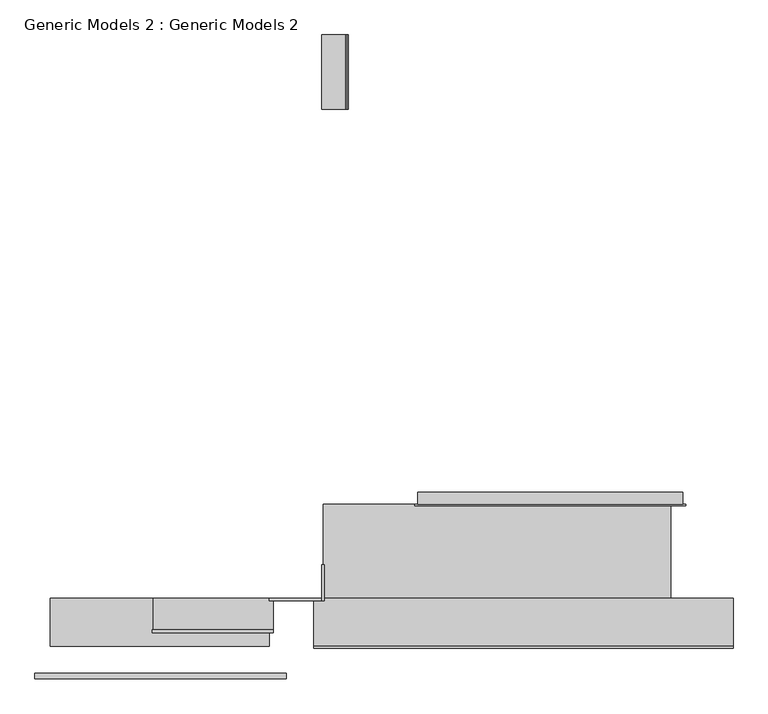
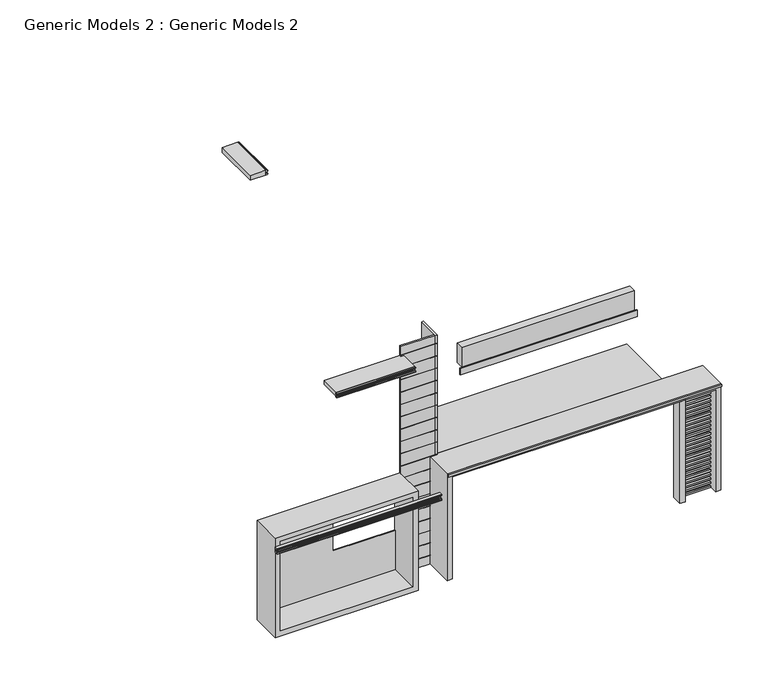
"""IFC4 building model written with IfcOpenShell, lengths in millimetres: proxy geometry, Generic Models 2 : Generic Models 2."""

from ifc_helpers import new_model, si_unit, point, frame, frame_2d, origin, place, context, project, spatial, polyline, circle_curve, trimmed, segment, composite_curve, outline, extrude, faceted_brep, source, transform, mapped, element, save


def generic_models_2_generic_models_2_638b9eba(model_context):
    return source(origin(), model_context, "Body", "SolidModel", [
        extrude(outline(polyline([(-7758.4277226, -3207.8444793), (-7758.4277226, -4630.2444793), (-7759.7175664, -4630.2444793), (-7759.7175664, -3207.8444793), (-7758.4277226, -3207.8444793)])), frame((0.0, 0.0, 6031.309375), z_axis=(0.0, 0.0, 1.0), x_axis=(1.0, 0.0, 0.0)), (0.0, 0.0, 1.0), 28.178125),
        extrude(outline(composite_curve([segment(polyline([(6121.4, -7759.7175664), (6059.4875, -7759.7175664), (6059.4875, -7747.0175664)]), True, "CONTINUOUS"), segment(trimmed(circle_curve(frame_2d((6072.1875, -7747.0175664)), 12.7), [point((6059.4875, -7747.0175664))], [point((6072.1875, -7734.3175664))], False, "CARTESIAN"), True, "CONTINUOUS"), segment(polyline([(6072.1875, -7734.3175664), (6083.3, -7734.3175664), (6083.3, -7708.9175664), (6102.35, -7708.9175664)]), True, "CONTINUOUS"), segment(trimmed(circle_curve(frame_2d((6102.35, -7727.9675664)), 19.05), [point((6102.35, -7708.9175664))], [point((6121.4, -7727.9675664))], False, "CARTESIAN"), True, "CONTINUOUS"), segment(polyline([(6121.4, -7727.9675664), (6121.4, -7759.7175664)]), True, "CONTINUOUS")], self_intersect=False)), frame((0.0, -4630.2444793, 0.0), z_axis=(0.0, 1.0, 0.0), x_axis=(0.0, 0.0, 1.0)), (0.0, 0.0, 1.0), 1422.4),
        extrude(outline(composite_curve([segment(polyline([(6031.309375, -7744.8133893), (6031.309375, -7759.7175664), (5969.396875, -7759.7175664), (5969.396875, -7727.9675664)]), True, "CONTINUOUS"), segment(trimmed(circle_curve(frame_2d((5988.446875, -7727.9675664)), 19.05), [point((5969.396875, -7727.9675664))], [point((5988.446875, -7708.9175664))], False, "CARTESIAN"), True, "CONTINUOUS"), segment(polyline([(5988.446875, -7708.9175664), (6007.496875, -7708.9175664), (6007.496875, -7734.3175664), (6020.8135521, -7734.3175664)]), True, "CONTINUOUS"), segment(trimmed(circle_curve(frame_2d((6020.8135521, -7744.8133893)), 10.4958229), [point((6020.8135521, -7734.3175664))], [point((6031.309375, -7744.8133893))], False, "CARTESIAN"), True, "CONTINUOUS")], self_intersect=False)), frame((0.0, -4630.2444793, 0.0), z_axis=(0.0, 1.0, 0.0), x_axis=(0.0, 0.0, 1.0)), (0.0, 0.0, 1.0), 1422.4),
        extrude(outline(polyline([(-7759.7175664, -3207.8444793), (-7759.7175664, -4630.2444793), (-8216.9175664, -4630.2444793), (-8216.9175664, -3207.8444793), (-7759.7175664, -3207.8444793)])), frame((0.0, 0.0, 5969.0), z_axis=(0.0, 0.0, 1.0), x_axis=(1.0, 0.0, 0.0)), (0.0, 0.0, 1.0), 152.4),
        extrude(outline(polyline([(-8891.4504606, -15389.4001854), (-13398.5175664, -15389.4001854), (-13398.5175664, -15388.1103416), (-8891.4504606, -15388.1103416), (-8891.4504606, -15389.4001854)])), frame((0.0, 0.0, 2971.7170487), z_axis=(0.0, 0.0, 1.0), x_axis=(1.0, 0.0, 0.0)), (0.0, 0.0, 1.0), 25.4),
        extrude(outline(polyline([(-6385.0131952, -11932.7444793), (-1334.7403048, -11932.7444793), (-1334.7403048, -12161.3444793), (-6385.0131952, -12161.3444793), (-6385.0131952, -11932.7444793)])), frame((0.0, 0.0, 4114.8), z_axis=(0.0, 0.0, 1.0), x_axis=(1.0, 0.0, 0.0)), (0.0, 0.0, 1.0), 609.6),
        extrude(outline(polyline([(-1269.5448198, -12186.7444793), (-6440.1403048, -12186.7444793), (-6440.1403048, -12161.3444793), (-1269.5448198, -12161.3444793), (-1269.5448198, -12186.7444793)])), frame((0.0, 0.0, 3909.9238233), z_axis=(0.0, 0.0, 1.0), x_axis=(1.0, 0.0, 0.0)), (0.0, 0.0, 1.0), 204.8761767),
        faceted_brep([(-8166.1175664, -14002.8444793, 3149.6), (-8166.1175664, -13313.1981155, 3149.6), (-8166.1175664, -13313.1981155, 6207.488841), (-8166.1175664, -14002.8444793, 6207.488841), (-8166.1175664, -14002.8444793, 5839.188841), (-8166.1175664, -13962.9992588, 5839.188841), (-8166.1175664, -13962.9992588, 5826.488841), (-8166.1175664, -14002.8444793, 5826.488841), (-8166.1175664, -14002.8444793, 5458.188841), (-8166.1175664, -13962.1298359, 5458.188841), (-8166.1175664, -13962.1298359, 5445.488841), (-8166.1175664, -14002.8444793, 5445.488841), (-8166.1175664, -14002.8444793, 5077.188841), (-8166.1175664, -13963.2783632, 5077.188841), (-8166.1175664, -13963.2783632, 5064.488841), (-8166.1175664, -14002.8444793, 5064.488841), (-8166.1175664, -14002.8444793, 4696.188841), (-8166.1175664, -13961.158785, 4696.188841), (-8166.1175664, -13961.158785, 4683.488841), (-8166.1175664, -14002.8444793, 4683.488841), (-8166.1175664, -14002.8444793, 4315.188841), (-8166.1175664, -13958.3944793, 4315.188841), (-8166.1175664, -13958.3944793, 4302.488841), (-8166.1175664, -14002.8444793, 4302.488841), (-8166.1175664, -14002.8444793, 3934.188841), (-8166.1175664, -13960.3451363, 3934.188841), (-8166.1175664, -13960.3451363, 3921.488841), (-8166.1175664, -14002.8444793, 3921.488841), (-8166.1175664, -14002.8444793, 3553.188841), (-8166.1175664, -13962.3673185, 3553.188841), (-8166.1175664, -13962.3673185, 3540.488841), (-8166.1175664, -14002.8444793, 3540.488841), (-8166.1175664, -14002.8444793, 3172.188841), (-8166.1175664, -13977.4444793, 3172.188841), (-8166.1175664, -13977.4444793, 3159.488841), (-8166.1175664, -14002.8444793, 3159.488841), (-8166.1175664, -13313.1981155, 6858.0), (-8166.1175664, -14002.8444793, 6858.0), (-8166.1175664, -14002.8444793, 6601.188841), (-8166.1175664, -13313.1981155, 6601.188841), (-8166.1175664, -13313.1981155, 6588.488841), (-8166.1175664, -14002.8444793, 6588.488841), (-8166.1175664, -14002.8444793, 6220.188841), (-8166.1175664, -13313.1981155, 6220.188841), (-8216.9175664, -14002.8444793, 6858.0), (-8216.9175664, -13313.1981155, 6858.0), (-8216.9175664, -13313.1981155, 3149.6), (-8216.9175664, -14002.8444793, 3149.6), (-8216.9175664, -14002.8444793, 3159.488841), (-8216.9175664, -13977.4444793, 3159.488841), (-8216.9175664, -13977.4444793, 3172.188841), (-8216.9175664, -14002.8444793, 3172.188841), (-8216.9175664, -14002.8444793, 3540.488841), (-8216.9175664, -13977.4444793, 3540.488841), (-8216.9175664, -13977.4444793, 3553.188841), (-8216.9175664, -14002.8444793, 3553.188841), (-8216.9175664, -14002.8444793, 3921.488841), (-8216.9175664, -13977.4444793, 3921.488841), (-8216.9175664, -13977.4444793, 3934.188841), (-8216.9175664, -14002.8444793, 3934.188841), (-8216.9175664, -14002.8444793, 4302.488841), (-8216.9175664, -13977.4444793, 4302.488841), (-8216.9175664, -13977.4444793, 4315.188841), (-8216.9175664, -14002.8444793, 4315.188841), (-8216.9175664, -14002.8444793, 4683.488841), (-8216.9175664, -13977.4444793, 4683.488841), (-8216.9175664, -13977.4444793, 4696.188841), (-8216.9175664, -14002.8444793, 4696.188841), (-8216.9175664, -14002.8444793, 5064.488841), (-8216.9175664, -13977.4444793, 5064.488841), (-8216.9175664, -13977.4444793, 5077.188841), (-8216.9175664, -14002.8444793, 5077.188841), (-8216.9175664, -14002.8444793, 5445.488841), (-8216.9175664, -13977.4444793, 5445.488841), (-8216.9175664, -13977.4444793, 5458.188841), (-8216.9175664, -14002.8444793, 5458.188841), (-8216.9175664, -14002.8444793, 5826.488841), (-8216.9175664, -13977.4444793, 5826.488841), (-8216.9175664, -13977.4444793, 5839.188841), (-8216.9175664, -14002.8444793, 5839.188841), (-8216.9175664, -14002.8444793, 6207.488841), (-8216.9175664, -13977.4444793, 6207.488841), (-8216.9175664, -13977.4444793, 6220.188841), (-8216.9175664, -14002.8444793, 6220.188841), (-8216.9175664, -14002.8444793, 6588.488841), (-8216.9175664, -13977.4444793, 6588.488841), (-8216.9175664, -13977.4444793, 6601.188841), (-8216.9175664, -14002.8444793, 6601.188841), (-8191.5175664, -13313.1981155, 6601.188841), (-8191.5175664, -13313.1981155, 6588.488841), (-8191.5175664, -13313.1981155, 6220.188841), (-8191.5175664, -13313.1981155, 6207.488841), (-8191.5175664, -13977.4444793, 3540.488841), (-8191.5175664, -13977.4444793, 3553.188841), (-8191.5175664, -13977.4444793, 3921.488841), (-8191.5175664, -13977.4444793, 3934.188841), (-8191.5175664, -13977.4444793, 4302.488841), (-8191.5175664, -13977.4444793, 4315.188841), (-8191.5175664, -13977.4444793, 4683.488841), (-8191.5175664, -13977.4444793, 4696.188841), (-8191.5175664, -13977.4444793, 5064.488841), (-8191.5175664, -13977.4444793, 5077.188841), (-8191.5175664, -13977.4444793, 5445.488841), (-8191.5175664, -13977.4444793, 5458.188841), (-8191.5175664, -13977.4444793, 5826.488841), (-8191.5175664, -13977.4444793, 5839.188841), (-8191.5175664, -13977.4444793, 6207.488841), (-8191.5175664, -13977.4444793, 6220.188841), (-8191.5175664, -13977.4444793, 6588.488841), (-8191.5175664, -13977.4444793, 6601.188841), (-8191.5175664, -13962.9992588, 5826.488841), (-8191.5175664, -13962.9992588, 5839.188841), (-8191.5175664, -13962.1298359, 5445.488841), (-8191.5175664, -13962.1298359, 5458.188841), (-8191.5175664, -13963.2783632, 5064.488841), (-8191.5175664, -13963.2783632, 5077.188841), (-8191.5175664, -13961.158785, 4683.488841), (-8191.5175664, -13961.158785, 4696.188841), (-8191.5175664, -13958.3944793, 4302.488841), (-8191.5175664, -13958.3944793, 4315.188841), (-8191.5175664, -13960.3451363, 3921.488841), (-8191.5175664, -13960.3451363, 3934.188841), (-8191.5175664, -13962.3673185, 3540.488841), (-8191.5175664, -13962.3673185, 3553.188841)], [[[0, 1, 2, 3, 4, 5, 6, 7, 8, 9, 10, 11, 12, 13, 14, 15, 16, 17, 18, 19, 20, 21, 22, 23, 24, 25, 26, 27, 28, 29, 30, 31, 32, 33, 34, 35]], [[36, 37, 38, 39]], [[40, 41, 42, 43]], [[44, 45, 46, 47, 48, 49, 50, 51, 52, 53, 54, 55, 56, 57, 58, 59, 60, 61, 62, 63, 64, 65, 66, 67, 68, 69, 70, 71, 72, 73, 74, 75, 76, 77, 78, 79, 80, 81, 82, 83, 84, 85, 86, 87]], [[1, 0, 47, 46]], [[46, 45, 36, 39, 88, 89, 40, 43, 90, 91, 2, 1]], [[37, 36, 45, 44]], [[4, 3, 80, 79]], [[8, 7, 76, 75]], [[12, 11, 72, 71]], [[16, 15, 68, 67]], [[20, 19, 64, 63]], [[24, 23, 60, 59]], [[28, 27, 56, 55]], [[32, 31, 52, 51]], [[42, 41, 84, 83]], [[47, 0, 35, 48]], [[37, 44, 87, 38]], [[54, 53, 92, 93]], [[58, 57, 94, 95]], [[62, 61, 96, 97]], [[66, 65, 98, 99]], [[70, 69, 100, 101]], [[74, 73, 102, 103]], [[78, 77, 104, 105]], [[82, 81, 106, 107]], [[86, 85, 108, 109]], [[33, 50, 49, 34]], [[40, 89, 108, 85, 84, 41]], [[38, 87, 86, 109, 88, 39]], [[2, 91, 106, 81, 80, 3]], [[42, 83, 82, 107, 90, 43]], [[6, 110, 104, 77, 76, 7]], [[4, 79, 78, 105, 111, 5]], [[10, 112, 102, 73, 72, 11]], [[8, 75, 74, 103, 113, 9]], [[14, 114, 100, 69, 68, 15]], [[12, 71, 70, 101, 115, 13]], [[18, 116, 98, 65, 64, 19]], [[16, 67, 66, 99, 117, 17]], [[22, 118, 96, 61, 60, 23]], [[20, 63, 62, 97, 119, 21]], [[26, 120, 94, 57, 56, 27]], [[24, 59, 58, 95, 121, 25]], [[30, 122, 92, 53, 52, 31]], [[28, 55, 54, 93, 123, 29]], [[34, 49, 48, 35]], [[50, 33, 32, 51]], [[108, 89, 88, 109]], [[106, 91, 90, 107]], [[104, 110, 111, 105]], [[102, 112, 113, 103]], [[100, 114, 115, 101]], [[98, 116, 117, 99]], [[96, 118, 119, 97]], [[94, 120, 121, 95]], [[92, 122, 123, 93]], [[111, 110, 6, 5]], [[113, 112, 10, 9]], [[115, 114, 14, 13]], [[117, 116, 18, 17]], [[119, 118, 22, 21]], [[121, 120, 26, 25]], [[123, 122, 30, 29]]]),
        faceted_brep([(-9220.2175664, -14002.8444793, -152.4), (-8369.3175664, -14002.8444793, -152.4), (-8369.3175664, -14002.8444793, 111.488841), (-9220.2175664, -14002.8444793, 111.488841), (-8369.3175664, -14002.8444793, 3149.6), (-8216.9175664, -14002.8444793, 3149.6), (-8216.9175664, -14002.8444793, 3159.488841), (-9220.2175664, -14002.8444793, 3159.488841), (-9220.2175664, -14002.8444793, 2791.188841), (-8369.3175664, -14002.8444793, 2791.188841), (-8216.9175664, -14002.8444793, 6858.0), (-9220.2175664, -14002.8444793, 6858.0), (-9220.2175664, -14002.8444793, 6601.188841), (-8216.9175664, -14002.8444793, 6601.188841), (-9220.2175664, -14002.8444793, 6588.488841), (-9220.2175664, -14002.8444793, 6220.188841), (-8216.9175664, -14002.8444793, 6220.188841), (-8216.9175664, -14002.8444793, 6588.488841), (-9220.2175664, -14002.8444793, 6207.488841), (-9220.2175664, -14002.8444793, 5839.188841), (-8216.9175664, -14002.8444793, 5839.188841), (-8216.9175664, -14002.8444793, 6207.488841), (-9220.2175664, -14002.8444793, 5826.488841), (-9220.2175664, -14002.8444793, 5458.188841), (-8216.9175664, -14002.8444793, 5458.188841), (-8216.9175664, -14002.8444793, 5826.488841), (-9220.2175664, -14002.8444793, 5445.488841), (-9220.2175664, -14002.8444793, 5077.188841), (-8216.9175664, -14002.8444793, 5077.188841), (-8216.9175664, -14002.8444793, 5445.488841), (-9220.2175664, -14002.8444793, 5064.488841), (-9220.2175664, -14002.8444793, 4696.188841), (-8216.9175664, -14002.8444793, 4696.188841), (-8216.9175664, -14002.8444793, 5064.488841), (-9220.2175664, -14002.8444793, 4683.488841), (-9220.2175664, -14002.8444793, 4315.188841), (-8216.9175664, -14002.8444793, 4315.188841), (-8216.9175664, -14002.8444793, 4683.488841), (-9220.2175664, -14002.8444793, 4302.488841), (-9220.2175664, -14002.8444793, 3934.188841), (-8216.9175664, -14002.8444793, 3934.188841), (-8216.9175664, -14002.8444793, 4302.488841), (-9220.2175664, -14002.8444793, 3921.488841), (-9220.2175664, -14002.8444793, 3553.188841), (-8216.9175664, -14002.8444793, 3553.188841), (-8216.9175664, -14002.8444793, 3921.488841), (-9220.2175664, -14002.8444793, 3540.488841), (-9220.2175664, -14002.8444793, 3172.188841), (-8216.9175664, -14002.8444793, 3172.188841), (-8216.9175664, -14002.8444793, 3540.488841), (-9220.2175664, -14002.8444793, 2778.488841), (-9220.2175664, -14002.8444793, 2410.188841), (-8369.3175664, -14002.8444793, 2410.188841), (-8369.3175664, -14002.8444793, 2778.488841), (-9220.2175664, -14002.8444793, 2397.488841), (-9220.2175664, -14002.8444793, 2029.188841), (-8369.3175664, -14002.8444793, 2029.188841), (-8369.3175664, -14002.8444793, 2397.488841), (-9220.2175664, -14002.8444793, 2016.488841), (-9220.2175664, -14002.8444793, 1648.188841), (-8369.3175664, -14002.8444793, 1648.188841), (-8369.3175664, -14002.8444793, 2016.488841), (-9220.2175664, -14002.8444793, 1635.488841), (-9220.2175664, -14002.8444793, 1267.188841), (-8369.3175664, -14002.8444793, 1267.188841), (-8369.3175664, -14002.8444793, 1635.488841), (-9220.2175664, -14002.8444793, 1254.488841), (-9220.2175664, -14002.8444793, 886.188841), (-8369.3175664, -14002.8444793, 886.188841), (-8369.3175664, -14002.8444793, 1254.488841), (-9220.2175664, -14002.8444793, 873.488841), (-9220.2175664, -14002.8444793, 505.188841), (-8369.3175664, -14002.8444793, 505.188841), (-8369.3175664, -14002.8444793, 873.488841), (-9220.2175664, -14002.8444793, 492.488841), (-9220.2175664, -14002.8444793, 124.188841), (-8369.3175664, -14002.8444793, 124.188841), (-8369.3175664, -14002.8444793, 492.488841), (-9220.2175664, -13952.0444793, 6858.0), (-8216.9175664, -13952.0444793, 6858.0), (-8216.9175664, -13952.0444793, 3149.6), (-8369.3175664, -13952.0444793, 3149.6), (-8369.3175664, -13952.0444793, -152.4), (-9220.2175664, -13952.0444793, -152.4), (-9220.2175664, -13977.4444793, 111.488841), (-9220.2175664, -13977.4444793, 124.188841), (-9220.2175664, -13977.4444793, 492.488841), (-9220.2175664, -13977.4444793, 505.188841), (-9220.2175664, -13977.4444793, 873.488841), (-9220.2175664, -13977.4444793, 886.188841), (-9220.2175664, -13977.4444793, 1254.488841), (-9220.2175664, -13977.4444793, 1267.188841), (-9220.2175664, -13977.4444793, 1635.488841), (-9220.2175664, -13977.4444793, 1648.188841), (-9220.2175664, -13977.4444793, 2016.488841), (-9220.2175664, -13977.4444793, 2029.188841), (-9220.2175664, -13977.4444793, 2397.488841), (-9220.2175664, -13977.4444793, 2410.188841), (-9220.2175664, -13977.4444793, 2778.488841), (-9220.2175664, -13977.4444793, 2791.188841), (-9220.2175664, -13977.4444793, 3159.488841), (-9220.2175664, -13977.4444793, 3172.188841), (-9220.2175664, -13977.4444793, 3540.488841), (-9220.2175664, -13977.4444793, 3553.188841), (-9220.2175664, -13977.4444793, 3921.488841), (-9220.2175664, -13977.4444793, 3934.188841), (-9220.2175664, -13977.4444793, 4302.488841), (-9220.2175664, -13977.4444793, 4315.188841), (-9220.2175664, -13977.4444793, 4683.488841), (-9220.2175664, -13977.4444793, 4696.188841), (-9220.2175664, -13977.4444793, 5064.488841), (-9220.2175664, -13977.4444793, 5077.188841), (-9220.2175664, -13977.4444793, 5445.488841), (-9220.2175664, -13977.4444793, 5458.188841), (-9220.2175664, -13977.4444793, 5826.488841), (-9220.2175664, -13977.4444793, 5839.188841), (-9220.2175664, -13977.4444793, 6207.488841), (-9220.2175664, -13977.4444793, 6220.188841), (-9220.2175664, -13977.4444793, 6588.488841), (-9220.2175664, -13977.4444793, 6601.188841), (-8369.3175664, -13977.4444793, 2791.188841), (-8369.3175664, -13977.4444793, 2778.488841), (-8369.3175664, -13977.4444793, 2410.188841), (-8369.3175664, -13977.4444793, 2397.488841), (-8369.3175664, -13977.4444793, 2029.188841), (-8369.3175664, -13977.4444793, 2016.488841), (-8369.3175664, -13977.4444793, 1648.188841), (-8369.3175664, -13977.4444793, 1635.488841), (-8369.3175664, -13977.4444793, 1267.188841), (-8369.3175664, -13977.4444793, 1254.488841), (-8369.3175664, -13977.4444793, 886.188841), (-8369.3175664, -13977.4444793, 873.488841), (-8369.3175664, -13977.4444793, 505.188841), (-8369.3175664, -13977.4444793, 492.488841), (-8369.3175664, -13977.4444793, 124.188841), (-8369.3175664, -13977.4444793, 111.488841), (-8216.9175664, -13977.4444793, 6601.188841), (-8216.9175664, -13977.4444793, 6588.488841), (-8216.9175664, -13977.4444793, 6220.188841), (-8216.9175664, -13977.4444793, 6207.488841), (-8216.9175664, -13977.4444793, 5839.188841), (-8216.9175664, -13977.4444793, 5826.488841), (-8216.9175664, -13977.4444793, 5458.188841), (-8216.9175664, -13977.4444793, 5445.488841), (-8216.9175664, -13977.4444793, 5077.188841), (-8216.9175664, -13977.4444793, 5064.488841), (-8216.9175664, -13977.4444793, 4696.188841), (-8216.9175664, -13977.4444793, 4683.488841), (-8216.9175664, -13977.4444793, 4315.188841), (-8216.9175664, -13977.4444793, 4302.488841), (-8216.9175664, -13977.4444793, 3934.188841), (-8216.9175664, -13977.4444793, 3921.488841), (-8216.9175664, -13977.4444793, 3553.188841), (-8216.9175664, -13977.4444793, 3540.488841), (-8216.9175664, -13977.4444793, 3172.188841), (-8216.9175664, -13977.4444793, 3159.488841)], [[[0, 1, 2, 3]], [[4, 5, 6, 7, 8, 9]], [[10, 11, 12, 13]], [[14, 15, 16, 17]], [[18, 19, 20, 21]], [[22, 23, 24, 25]], [[26, 27, 28, 29]], [[30, 31, 32, 33]], [[34, 35, 36, 37]], [[38, 39, 40, 41]], [[42, 43, 44, 45]], [[46, 47, 48, 49]], [[50, 51, 52, 53]], [[54, 55, 56, 57]], [[58, 59, 60, 61]], [[62, 63, 64, 65]], [[66, 67, 68, 69]], [[70, 71, 72, 73]], [[74, 75, 76, 77]], [[78, 79, 80, 81, 82, 83]], [[78, 83, 0, 3, 84, 85, 75, 74, 86, 87, 71, 70, 88, 89, 67, 66, 90, 91, 63, 62, 92, 93, 59, 58, 94, 95, 55, 54, 96, 97, 51, 50, 98, 99, 8, 7, 100, 101, 47, 46, 102, 103, 43, 42, 104, 105, 39, 38, 106, 107, 35, 34, 108, 109, 31, 30, 110, 111, 27, 26, 112, 113, 23, 22, 114, 115, 19, 18, 116, 117, 15, 14, 118, 119, 12, 11]], [[1, 0, 83, 82]], [[82, 81, 4, 9, 120, 121, 53, 52, 122, 123, 57, 56, 124, 125, 61, 60, 126, 127, 65, 64, 128, 129, 69, 68, 130, 131, 73, 72, 132, 133, 77, 76, 134, 135, 2, 1]], [[5, 4, 81, 80]], [[80, 79, 10, 13, 136, 137, 17, 16, 138, 139, 21, 20, 140, 141, 25, 24, 142, 143, 29, 28, 144, 145, 33, 32, 146, 147, 37, 36, 148, 149, 41, 40, 150, 151, 45, 44, 152, 153, 49, 48, 154, 155, 6, 5]], [[11, 10, 79, 78]], [[136, 119, 118, 137]], [[138, 117, 116, 139]], [[140, 115, 114, 141]], [[142, 113, 112, 143]], [[144, 111, 110, 145]], [[146, 109, 108, 147]], [[148, 107, 106, 149]], [[150, 105, 104, 151]], [[152, 103, 102, 153]], [[154, 101, 100, 155]], [[120, 99, 98, 121]], [[122, 97, 96, 123]], [[124, 95, 94, 125]], [[126, 93, 92, 127]], [[128, 91, 90, 129]], [[130, 89, 88, 131]], [[132, 87, 86, 133]], [[134, 85, 84, 135]], [[137, 118, 14, 17]], [[119, 136, 13, 12]], [[139, 116, 18, 21]], [[117, 138, 16, 15]], [[141, 114, 22, 25]], [[115, 140, 20, 19]], [[143, 112, 26, 29]], [[113, 142, 24, 23]], [[145, 110, 30, 33]], [[111, 144, 28, 27]], [[147, 108, 34, 37]], [[109, 146, 32, 31]], [[149, 106, 38, 41]], [[107, 148, 36, 35]], [[151, 104, 42, 45]], [[105, 150, 40, 39]], [[153, 102, 46, 49]], [[103, 152, 44, 43]], [[155, 100, 7, 6]], [[101, 154, 48, 47]], [[121, 98, 50, 53]], [[99, 120, 9, 8]], [[123, 96, 54, 57]], [[97, 122, 52, 51]], [[125, 94, 58, 61]], [[95, 124, 56, 55]], [[127, 92, 62, 65]], [[93, 126, 60, 59]], [[129, 90, 66, 69]], [[91, 128, 64, 63]], [[131, 88, 70, 73]], [[89, 130, 68, 67]], [[133, 86, 74, 77]], [[87, 132, 72, 71]], [[135, 84, 3, 2]], [[85, 134, 76, 75]]]),
        extrude(outline(polyline([(-152.4, -9220.2175664), (2921.0, -9220.2175664), (2921.0, -13398.5175664), (-152.4, -13398.5175664), (-152.4, -9220.2175664)]), holes=[polyline([(2768.6, -13246.1175664), (2768.6, -9372.6175664), (0.0, -9372.6175664), (0.0, -13246.1175664), (2768.6, -13246.1175664)])]), frame((0.0, -14866.4444793, 0.0), z_axis=(0.0, 1.0, 0.0), x_axis=(0.0, 0.0, 1.0)), (0.0, 0.0, 1.0), 914.4),
        extrude(outline(composite_curve([segment(polyline([(-14587.0444793, 6528.1165597), (-14595.3522225, 6528.1165597)]), True, "CONTINUOUS"), segment(trimmed(circle_curve(frame_2d((-14595.3522225, 6545.2088165)), 17.0922568), [point((-14595.3522225, 6528.1165597))], [point((-14612.4444793, 6545.2088165))], False, "CARTESIAN"), True, "CONTINUOUS"), segment(polyline([(-14612.4444793, 6545.2088165), (-14612.4444793, 6553.8331194), (-14561.6444793, 6553.8331194), (-14561.6444793, 6509.0665597), (-14571.1956144, 6509.0665597)]), True, "CONTINUOUS"), segment(trimmed(circle_curve(frame_2d((-14571.1956144, 6524.9154246)), 15.8488649), [point((-14571.1956144, 6509.0665597))], [point((-14587.0444793, 6524.9154246))], False, "CARTESIAN"), True, "CONTINUOUS"), segment(polyline([(-14587.0444793, 6524.9154246), (-14587.0444793, 6528.1165597)]), True, "CONTINUOUS")], self_intersect=False)), frame((-11455.4175664, 0.0, 0.0), z_axis=(1.0, 0.0, 0.0), x_axis=(0.0, 1.0, 0.0)), (0.0, 0.0, 1.0), 2311.4),
        extrude(outline(composite_curve([segment(polyline([(-14587.0444793, 6451.9165597), (-14587.0444793, 6458.2665597)]), True, "CONTINUOUS"), segment(trimmed(circle_curve(frame_2d((-14574.3444793, 6458.2665597)), 12.7), [point((-14587.0444793, 6458.2665597))], [point((-14574.3444793, 6470.9665597))], False, "CARTESIAN"), True, "CONTINUOUS"), segment(polyline([(-14574.3444793, 6470.9665597), (-14561.6444793, 6470.9665597), (-14561.6444793, 6426.2), (-14612.4444793, 6426.2), (-14612.4444793, 6435.88805)]), True, "CONTINUOUS"), segment(trimmed(circle_curve(frame_2d((-14596.4159696, 6435.88805)), 16.0285097), [point((-14612.4444793, 6435.88805))], [point((-14596.4159696, 6451.9165597))], False, "CARTESIAN"), True, "CONTINUOUS"), segment(polyline([(-14596.4159696, 6451.9165597), (-14587.0444793, 6451.9165597)]), True, "CONTINUOUS")], self_intersect=False)), frame((-11455.4175664, 0.0, 0.0), z_axis=(1.0, 0.0, 0.0), x_axis=(0.0, 1.0, 0.0)), (0.0, 0.0, 1.0), 2311.4),
        extrude(outline(polyline([(-9144.0175664, -14561.6444793), (-11430.0175664, -14561.6444793), (-11430.0175664, -13952.0444793), (-9144.0175664, -13952.0444793), (-9144.0175664, -14561.6444793)])), frame((0.0, 0.0, 6426.2), z_axis=(0.0, 0.0, 1.0), x_axis=(1.0, 0.0, 0.0)), (0.0, 0.0, 1.0), 127.6331194),
        extrude(outline(polyline([(-1408.2775173, -14631.4944793), (-1408.2775173, -14561.6444793), (-521.9403048, -14561.6444793), (-521.9403048, -14631.4944793), (-1408.2775173, -14631.4944793)])), frame((0.0, 0.0, 2881.5099842), z_axis=(0.0, 0.0, 1.0), x_axis=(1.0, 0.0, 0.0)), (0.0, 0.0, 1.0), 115.6900158),
        extrude(outline(polyline([(-1408.2775173, -14631.4944793), (-1408.2775173, -14561.6444793), (-521.9403048, -14561.6444793), (-521.9403048, -14631.4944793), (-1408.2775173, -14631.4944793)])), frame((0.0, 0.0, -152.4), z_axis=(0.0, 0.0, 1.0), x_axis=(1.0, 0.0, 0.0)), (0.0, 0.0, 1.0), 36.7099842),
        extrude(outline(polyline([(-1408.2775173, -14631.4944793), (-1408.2775173, -14561.6444793), (-521.9403048, -14561.6444793), (-521.9403048, -14631.4944793), (-1408.2775173, -14631.4944793)])), frame((0.0, 0.0, 2754.5099842), z_axis=(0.0, 0.0, 1.0), x_axis=(1.0, 0.0, 0.0)), (0.0, 0.0, 1.0), 50.8),
        extrude(outline(polyline([(-1408.2775173, -14631.4944793), (-1408.2775173, -14561.6444793), (-521.9403048, -14561.6444793), (-521.9403048, -14631.4944793), (-1408.2775173, -14631.4944793)])), frame((0.0, 0.0, 2627.5099842), z_axis=(0.0, 0.0, 1.0), x_axis=(1.0, 0.0, 0.0)), (0.0, 0.0, 1.0), 50.8),
        extrude(outline(polyline([(-1408.2775173, -14631.4944793), (-1408.2775173, -14561.6444793), (-521.9403048, -14561.6444793), (-521.9403048, -14631.4944793), (-1408.2775173, -14631.4944793)])), frame((0.0, 0.0, 2500.5099842), z_axis=(0.0, 0.0, 1.0), x_axis=(1.0, 0.0, 0.0)), (0.0, 0.0, 1.0), 50.8),
        extrude(outline(polyline([(-1408.2775173, -14631.4944793), (-1408.2775173, -14561.6444793), (-521.9403048, -14561.6444793), (-521.9403048, -14631.4944793), (-1408.2775173, -14631.4944793)])), frame((0.0, 0.0, 2373.5099842), z_axis=(0.0, 0.0, 1.0), x_axis=(1.0, 0.0, 0.0)), (0.0, 0.0, 1.0), 50.8),
        extrude(outline(polyline([(-1408.2775173, -14631.4944793), (-1408.2775173, -14561.6444793), (-521.9403048, -14561.6444793), (-521.9403048, -14631.4944793), (-1408.2775173, -14631.4944793)])), frame((0.0, 0.0, 2246.5099842), z_axis=(0.0, 0.0, 1.0), x_axis=(1.0, 0.0, 0.0)), (0.0, 0.0, 1.0), 50.8),
        extrude(outline(polyline([(-1408.2775173, -14631.4944793), (-1408.2775173, -14561.6444793), (-521.9403048, -14561.6444793), (-521.9403048, -14631.4944793), (-1408.2775173, -14631.4944793)])), frame((0.0, 0.0, 2119.5099842), z_axis=(0.0, 0.0, 1.0), x_axis=(1.0, 0.0, 0.0)), (0.0, 0.0, 1.0), 50.8),
        extrude(outline(polyline([(-1408.2775173, -14631.4944793), (-1408.2775173, -14561.6444793), (-521.9403048, -14561.6444793), (-521.9403048, -14631.4944793), (-1408.2775173, -14631.4944793)])), frame((0.0, 0.0, 1992.5099842), z_axis=(0.0, 0.0, 1.0), x_axis=(1.0, 0.0, 0.0)), (0.0, 0.0, 1.0), 50.8),
        extrude(outline(polyline([(-1408.2775173, -14631.4944793), (-1408.2775173, -14561.6444793), (-521.9403048, -14561.6444793), (-521.9403048, -14631.4944793), (-1408.2775173, -14631.4944793)])), frame((0.0, 0.0, 1865.5099842), z_axis=(0.0, 0.0, 1.0), x_axis=(1.0, 0.0, 0.0)), (0.0, 0.0, 1.0), 50.8),
        extrude(outline(polyline([(-1408.2775173, -14631.4944793), (-1408.2775173, -14561.6444793), (-521.9403048, -14561.6444793), (-521.9403048, -14631.4944793), (-1408.2775173, -14631.4944793)])), frame((0.0, 0.0, 1738.5099842), z_axis=(0.0, 0.0, 1.0), x_axis=(1.0, 0.0, 0.0)), (0.0, 0.0, 1.0), 50.8),
        extrude(outline(polyline([(-1408.2775173, -14631.4944793), (-1408.2775173, -14561.6444793), (-521.9403048, -14561.6444793), (-521.9403048, -14631.4944793), (-1408.2775173, -14631.4944793)])), frame((0.0, 0.0, 1611.5099842), z_axis=(0.0, 0.0, 1.0), x_axis=(1.0, 0.0, 0.0)), (0.0, 0.0, 1.0), 50.8),
        extrude(outline(polyline([(-1408.2775173, -14631.4944793), (-1408.2775173, -14561.6444793), (-521.9403048, -14561.6444793), (-521.9403048, -14631.4944793), (-1408.2775173, -14631.4944793)])), frame((0.0, 0.0, 1484.5099842), z_axis=(0.0, 0.0, 1.0), x_axis=(1.0, 0.0, 0.0)), (0.0, 0.0, 1.0), 50.8),
        extrude(outline(polyline([(-1408.2775173, -14631.4944793), (-1408.2775173, -14561.6444793), (-521.9403048, -14561.6444793), (-521.9403048, -14631.4944793), (-1408.2775173, -14631.4944793)])), frame((0.0, 0.0, 1357.5099842), z_axis=(0.0, 0.0, 1.0), x_axis=(1.0, 0.0, 0.0)), (0.0, 0.0, 1.0), 50.8),
        extrude(outline(polyline([(-1408.2775173, -14631.4944793), (-1408.2775173, -14561.6444793), (-521.9403048, -14561.6444793), (-521.9403048, -14631.4944793), (-1408.2775173, -14631.4944793)])), frame((0.0, 0.0, 1230.5099842), z_axis=(0.0, 0.0, 1.0), x_axis=(1.0, 0.0, 0.0)), (0.0, 0.0, 1.0), 50.8),
        extrude(outline(polyline([(-1408.2775173, -14631.4944793), (-1408.2775173, -14561.6444793), (-521.9403048, -14561.6444793), (-521.9403048, -14631.4944793), (-1408.2775173, -14631.4944793)])), frame((0.0, 0.0, 1103.5099842), z_axis=(0.0, 0.0, 1.0), x_axis=(1.0, 0.0, 0.0)), (0.0, 0.0, 1.0), 50.8),
        extrude(outline(polyline([(-1408.2775173, -14631.4944793), (-1408.2775173, -14561.6444793), (-521.9403048, -14561.6444793), (-521.9403048, -14631.4944793), (-1408.2775173, -14631.4944793)])), frame((0.0, 0.0, 976.5099842), z_axis=(0.0, 0.0, 1.0), x_axis=(1.0, 0.0, 0.0)), (0.0, 0.0, 1.0), 50.8),
        extrude(outline(polyline([(-1408.2775173, -14631.4944793), (-1408.2775173, -14561.6444793), (-521.9403048, -14561.6444793), (-521.9403048, -14631.4944793), (-1408.2775173, -14631.4944793)])), frame((0.0, 0.0, 849.5099842), z_axis=(0.0, 0.0, 1.0), x_axis=(1.0, 0.0, 0.0)), (0.0, 0.0, 1.0), 50.8),
        extrude(outline(polyline([(-1408.2775173, -14631.4944793), (-1408.2775173, -14561.6444793), (-521.9403048, -14561.6444793), (-521.9403048, -14631.4944793), (-1408.2775173, -14631.4944793)])), frame((0.0, 0.0, 722.5099842), z_axis=(0.0, 0.0, 1.0), x_axis=(1.0, 0.0, 0.0)), (0.0, 0.0, 1.0), 50.8),
        extrude(outline(polyline([(-1408.2775173, -14631.4944793), (-1408.2775173, -14561.6444793), (-521.9403048, -14561.6444793), (-521.9403048, -14631.4944793), (-1408.2775173, -14631.4944793)])), frame((0.0, 0.0, 595.5099842), z_axis=(0.0, 0.0, 1.0), x_axis=(1.0, 0.0, 0.0)), (0.0, 0.0, 1.0), 50.8),
        extrude(outline(polyline([(-1408.2775173, -14631.4944793), (-1408.2775173, -14561.6444793), (-521.9403048, -14561.6444793), (-521.9403048, -14631.4944793), (-1408.2775173, -14631.4944793)])), frame((0.0, 0.0, 468.5099842), z_axis=(0.0, 0.0, 1.0), x_axis=(1.0, 0.0, 0.0)), (0.0, 0.0, 1.0), 50.8),
        extrude(outline(polyline([(-1408.2775173, -14631.4944793), (-1408.2775173, -14561.6444793), (-521.9403048, -14561.6444793), (-521.9403048, -14631.4944793), (-1408.2775173, -14631.4944793)])), frame((0.0, 0.0, 341.5099842), z_axis=(0.0, 0.0, 1.0), x_axis=(1.0, 0.0, 0.0)), (0.0, 0.0, 1.0), 50.8),
        extrude(outline(polyline([(-1408.2775173, -14631.4944793), (-1408.2775173, -14561.6444793), (-521.9403048, -14561.6444793), (-521.9403048, -14631.4944793), (-1408.2775173, -14631.4944793)])), frame((0.0, 0.0, 214.5099842), z_axis=(0.0, 0.0, 1.0), x_axis=(1.0, 0.0, 0.0)), (0.0, 0.0, 1.0), 50.8),
        extrude(outline(polyline([(-1408.2775173, -14631.4944793), (-1408.2775173, -14561.6444793), (-521.9403048, -14561.6444793), (-521.9403048, -14631.4944793), (-1408.2775173, -14631.4944793)])), frame((0.0, 0.0, 87.5099842), z_axis=(0.0, 0.0, 1.0), x_axis=(1.0, 0.0, 0.0)), (0.0, 0.0, 1.0), 50.8),
        extrude(outline(polyline([(-1408.2775173, -14631.4944793), (-1408.2775173, -14561.6444793), (-521.9403048, -14561.6444793), (-521.9403048, -14631.4944793), (-1408.2775173, -14631.4944793)])), frame((0.0, 0.0, -39.4900158), z_axis=(0.0, 0.0, 1.0), x_axis=(1.0, 0.0, 0.0)), (0.0, 0.0, 1.0), 50.8),
        extrude(outline(polyline([(-1563.3403048, -14866.4444793), (-1563.3403048, -14561.6444793), (-1408.2775173, -14561.6444793), (-1408.2775173, -14866.4444793), (-1563.3403048, -14866.4444793)])), frame((0.0, 0.0, -152.4), z_axis=(0.0, 0.0, 1.0), x_axis=(1.0, 0.0, 0.0)), (0.0, 0.0, 1.0), 3149.6),
        faceted_brep([(-8216.9175664, -14866.4444793, -152.4), (-8216.9175664, -14866.4444793, 2997.2), (-521.9403048, -14866.4444793, 2997.2), (-521.9403048, -14866.4444793, -152.4), (-369.5403048, -14866.4444793, -152.4), (-369.5403048, -14866.4444793, 3149.6), (-8369.3175664, -14866.4444793, 3149.6), (-8369.3175664, -14866.4444793, -152.4), (-8216.9175664, -13952.0444793, -152.4), (-8369.3175664, -13952.0444793, -152.4), (-8369.3175664, -13952.0444793, 3149.6), (-369.5403048, -13952.0444793, 3149.6), (-369.5403048, -13952.0444793, -152.4), (-521.9403048, -13952.0444793, -152.4), (-521.9403048, -13952.0444793, 2997.2), (-8216.9175664, -13952.0444793, 2997.2), (-8216.9175664, -13977.4444793, 2791.188841), (-8216.9175664, -13977.4444793, 2778.488841), (-8216.9175664, -14002.8444793, 2778.488841), (-8216.9175664, -14002.8444793, 2791.188841), (-8216.9175664, -13977.4444793, 2410.188841), (-8216.9175664, -13977.4444793, 2397.488841), (-8216.9175664, -14002.8444793, 2397.488841), (-8216.9175664, -14002.8444793, 2410.188841), (-8216.9175664, -13977.4444793, 2029.188841), (-8216.9175664, -13977.4444793, 2016.488841), (-8216.9175664, -14002.8444793, 2016.488841), (-8216.9175664, -14002.8444793, 2029.188841), (-8216.9175664, -13977.4444793, 1648.188841), (-8216.9175664, -13977.4444793, 1635.488841), (-8216.9175664, -14002.8444793, 1635.488841), (-8216.9175664, -14002.8444793, 1648.188841), (-8216.9175664, -13977.4444793, 1267.188841), (-8216.9175664, -13977.4444793, 1254.488841), (-8216.9175664, -14002.8444793, 1254.488841), (-8216.9175664, -14002.8444793, 1267.188841), (-8216.9175664, -13977.4444793, 886.188841), (-8216.9175664, -13977.4444793, 873.488841), (-8216.9175664, -14002.8444793, 873.488841), (-8216.9175664, -14002.8444793, 886.188841), (-8216.9175664, -13977.4444793, 505.188841), (-8216.9175664, -13977.4444793, 492.488841), (-8216.9175664, -14002.8444793, 492.488841), (-8216.9175664, -14002.8444793, 505.188841), (-8216.9175664, -13977.4444793, 124.188841), (-8216.9175664, -13977.4444793, 111.488841), (-8216.9175664, -14002.8444793, 111.488841), (-8216.9175664, -14002.8444793, 124.188841), (-8369.3175664, -13977.4444793, 2778.488841), (-8369.3175664, -13977.4444793, 2791.188841), (-8369.3175664, -14002.8444793, 2791.188841), (-8369.3175664, -14002.8444793, 2778.488841), (-8369.3175664, -13977.4444793, 2397.488841), (-8369.3175664, -13977.4444793, 2410.188841), (-8369.3175664, -14002.8444793, 2410.188841), (-8369.3175664, -14002.8444793, 2397.488841), (-8369.3175664, -13977.4444793, 2016.488841), (-8369.3175664, -13977.4444793, 2029.188841), (-8369.3175664, -14002.8444793, 2029.188841), (-8369.3175664, -14002.8444793, 2016.488841), (-8369.3175664, -13977.4444793, 1635.488841), (-8369.3175664, -13977.4444793, 1648.188841), (-8369.3175664, -14002.8444793, 1648.188841), (-8369.3175664, -14002.8444793, 1635.488841), (-8369.3175664, -13977.4444793, 1254.488841), (-8369.3175664, -13977.4444793, 1267.188841), (-8369.3175664, -14002.8444793, 1267.188841), (-8369.3175664, -14002.8444793, 1254.488841), (-8369.3175664, -13977.4444793, 873.488841), (-8369.3175664, -13977.4444793, 886.188841), (-8369.3175664, -14002.8444793, 886.188841), (-8369.3175664, -14002.8444793, 873.488841), (-8369.3175664, -13977.4444793, 492.488841), (-8369.3175664, -13977.4444793, 505.188841), (-8369.3175664, -14002.8444793, 505.188841), (-8369.3175664, -14002.8444793, 492.488841), (-8369.3175664, -13977.4444793, 111.488841), (-8369.3175664, -13977.4444793, 124.188841), (-8369.3175664, -14002.8444793, 124.188841), (-8369.3175664, -14002.8444793, 111.488841)], [[[0, 1, 2, 3, 4, 5, 6, 7]], [[8, 9, 10, 11, 12, 13, 14, 15]], [[1, 0, 8, 15], [16, 17, 18, 19], [20, 21, 22, 23], [24, 25, 26, 27], [28, 29, 30, 31], [32, 33, 34, 35], [36, 37, 38, 39], [40, 41, 42, 43], [44, 45, 46, 47]], [[2, 1, 15, 14]], [[3, 2, 14, 13]], [[4, 3, 13, 12]], [[5, 4, 12, 11]], [[6, 5, 11, 10]], [[7, 6, 10, 9], [48, 49, 50, 51], [52, 53, 54, 55], [56, 57, 58, 59], [60, 61, 62, 63], [64, 65, 66, 67], [68, 69, 70, 71], [72, 73, 74, 75], [76, 77, 78, 79]], [[0, 7, 9, 8]], [[16, 49, 48, 17]], [[20, 53, 52, 21]], [[24, 57, 56, 25]], [[28, 61, 60, 29]], [[32, 65, 64, 33]], [[36, 69, 68, 37]], [[40, 73, 72, 41]], [[44, 77, 76, 45]], [[18, 51, 50, 19]], [[22, 55, 54, 23]], [[26, 59, 58, 27]], [[30, 63, 62, 31]], [[34, 67, 66, 35]], [[38, 71, 70, 39]], [[42, 75, 74, 43]], [[46, 79, 78, 47]], [[17, 48, 51, 18]], [[49, 16, 19, 50]], [[21, 52, 55, 22]], [[53, 20, 23, 54]], [[25, 56, 59, 26]], [[57, 24, 27, 58]], [[29, 60, 63, 30]], [[61, 28, 31, 62]], [[33, 64, 67, 34]], [[65, 32, 35, 66]], [[37, 68, 71, 38]], [[69, 36, 39, 70]], [[41, 72, 75, 42]], [[73, 40, 43, 74]], [[45, 76, 79, 46]], [[77, 44, 47, 78]]]),
        extrude(outline(polyline([(-8184.4132689, -12161.3444793), (-1563.3403048, -12161.3444793), (-1563.3403048, -13952.0444793), (-8184.4132689, -13952.0444793), (-8184.4132689, -12161.3444793)])), frame((0.0, 0.0, 2997.2), z_axis=(0.0, 0.0, 1.0), x_axis=(1.0, 0.0, 0.0)), (0.0, 0.0, 1.0), 152.4),
        extrude(outline(composite_curve([segment(polyline([(-15388.1103416, 2997.1170487), (-15413.5103416, 2997.1170487), (-15413.5103416, 3009.8170487), (-15454.1503416, 3009.8170487)]), True, "CONTINUOUS"), segment(trimmed(circle_curve(frame_2d((-15454.1503416, 3019.9770487)), 10.16), [point((-15454.1503416, 3009.8170487))], [point((-15464.3103416, 3019.9770487))], False, "CARTESIAN"), True, "CONTINUOUS"), segment(polyline([(-15464.3103416, 3019.9770487), (-15464.3103416, 3035.2170487), (-15477.0103416, 3035.2170487)]), True, "CONTINUOUS"), segment(trimmed(circle_curve(frame_2d((-15477.0103416, 3047.9170487)), 12.7), [point((-15477.0103416, 3035.2170487))], [point((-15489.7103416, 3047.9170487))], False, "CARTESIAN"), True, "CONTINUOUS"), segment(polyline([(-15489.7103416, 3047.9170487), (-15489.7103416, 3073.2340973), (-15388.1103416, 3073.2340973), (-15388.1103416, 2997.1170487)]), True, "CONTINUOUS")], self_intersect=False)), frame((-13690.4629606, 0.0, 0.0), z_axis=(1.0, 0.0, 0.0), x_axis=(0.0, 1.0, 0.0)), (0.0, 0.0, 1.0), 4799.0125),
        extrude(outline(composite_curve([segment(polyline([(-15388.1103416, 2971.7170487), (-15388.1103416, 2895.6), (-15489.7103416, 2895.6), (-15489.7103416, 2920.9170487)]), True, "CONTINUOUS"), segment(trimmed(circle_curve(frame_2d((-15477.0103416, 2920.9170487)), 12.7), [point((-15489.7103416, 2920.9170487))], [point((-15477.0103416, 2933.6170487))], False, "CARTESIAN"), True, "CONTINUOUS"), segment(polyline([(-15477.0103416, 2933.6170487), (-15464.3103416, 2933.6170487), (-15464.3103416, 2948.8570487)]), True, "CONTINUOUS"), segment(trimmed(circle_curve(frame_2d((-15454.1503416, 2948.8570487)), 10.16), [point((-15464.3103416, 2948.8570487))], [point((-15454.1503416, 2959.0170487))], False, "CARTESIAN"), True, "CONTINUOUS"), segment(polyline([(-15454.1503416, 2959.0170487), (-15413.5103416, 2959.0170487), (-15413.5103416, 2971.7170487), (-15388.1103416, 2971.7170487)]), True, "CONTINUOUS")], self_intersect=False)), frame((-13690.4629606, 0.0, 0.0), z_axis=(1.0, 0.0, 0.0), x_axis=(0.0, 1.0, 0.0)), (0.0, 0.0, 1.0), 4799.0125),
        extrude(outline(polyline([(-8369.3175664, -14914.0694793), (-8369.3175664, -14866.4444793), (-369.5403048, -14866.4444793), (-369.5403048, -14914.0694793), (-8369.3175664, -14914.0694793)])), frame((0.0, 0.0, 3076.575), z_axis=(0.0, 0.0, 1.0), x_axis=(1.0, 0.0, 0.0)), (0.0, 0.0, 1.0), 73.025),
        extrude(outline(polyline([(1219.2, -11201.4175664), (2768.6, -11201.4175664), (2768.6, -13246.1175664), (0.0, -13246.1175664), (0.0, -9372.6175664), (1219.2, -9372.6175664), (1219.2, -11201.4175664)])), frame((0.0, -13977.4444793, 0.0), z_axis=(0.0, 1.0, 0.0), x_axis=(0.0, 0.0, 1.0)), (0.0, 0.0, 1.0), 25.4),
    ])


if __name__ == "__main__":
    model = new_model("IFC4")
    model_context = context("Model", 3, world=origin())
    ifc_project = project(units=[si_unit("LENGTHUNIT", "METRE", prefix="MILLI")], contexts=[model_context])
    site = spatial("IfcSite", under=ifc_project)
    building = spatial("IfcBuilding", under=site)
    placement = place(None, origin())
    generic_models_2_generic_models_2_shape = generic_models_2_generic_models_2_638b9eba(model_context)
    element("IfcBuildingElementProxy", 1, Name="Generic Models 2 : Generic Models 2", ObjectType="Generic Models 2 : Generic Models 2", at=placement, inside=building, context=model_context, shape_type="MappedRepresentation", body=[
        mapped(generic_models_2_generic_models_2_shape, transform((0.0, 0.0, 0.0), x_axis=(1.0, 0.0, 0.0), y_axis=(0.0, 1.0, 0.0), z_axis=(0.0, 0.0, 1.0))),
    ])
    save(model, "model.ifc")

# Revit data of these elements
# Element 1 (IfcBuildingElementProxy, "Generic Models 2 : Generic Models 2")
#   Materials on its faces: "Gypsum Wall Board", "Damp-proofing", "Laminate, Ivory, Matte", "window wall", "wood balcony"
# Materials
#   "Gypsum Wall Board": class "Generic", colour RGB 127 127 127, transparency 0, Description = "Gypsum Wall Board", Cost = 0
#   "Damp-proofing": class "Generic", colour RGB 127 127 127, transparency 0, Description = "Damp-proofing", Cost = 0
#   "Laminate, Ivory, Matte": class "Plastic", colour RGB 247 247 239, transparency 0, Description = "Plastic Laminate - Ivory, Matte", Cost = 0
#   "window wall": class "Generic", colour RGB 120 120 120, transparency 0, Cost = 0
#   "wood balcony": class "Generic", colour RGB 120 120 120, transparency 0, Cost = 0
